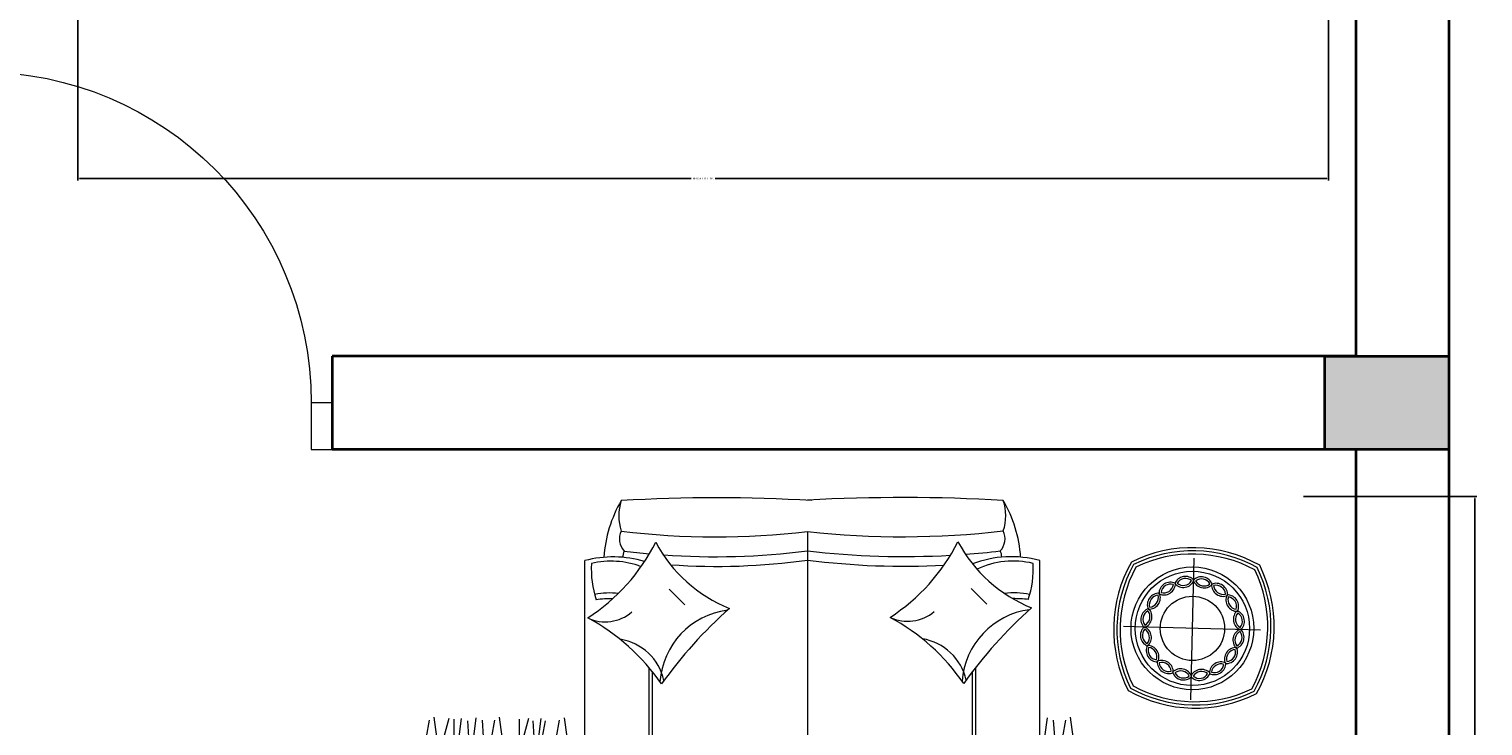
# Model space of a CAD drawing. Units: inches. Extents: x 1602 to 2642, y 1463 to 2270.
# Tile 3 of 5: x 1854 to 1995, y 1851 to 1919. Entities that reach past the tile are written whole.
import ezdxf

# ---------------------------------------------------------------- set-up
doc = ezdxf.new("R2010")
doc.units = ezdxf.units.IN
for name, color, linetype, lineweight in [('A-ANNO-DIMS', 2, 'Continuous', 18), ('A-COLS', 7, 'Continuous', 35), ('A-DOOR', 3, 'Continuous', 18), ('A-FURN', 8, 'Continuous', 13), ('A-WALL', 7, 'Continuous', 35)]:
    doc.layers.add(name, color=color, linetype=linetype, lineweight=lineweight)
doc.styles.get("Standard").update_dxf_attribs({"font": 'arial.ttf'})
doc.dimstyles.get("Standard").update_dxf_attribs({"dimtxt": 0.18, "dimasz": 0.18, "dimexe": 0.18, "dimexo": 0.0625, "dimgap": 0.09, "dimtad": 0, "dimtih": 1, "dimtoh": 1, "dimdec": 4, "dimzin": 0, "dimdsep": 46, "dimtxsty": 'Standard', "dimcen": 0.09, "dimadec": 0, "dimazin": 0, "dimtfac": 1, "dimtdec": 4, "dimtofl": 0, "dimtmove": 0, "dimatfit": 3, "dimfxl": 1, "dimtolj": 1, "dimtzin": 0, "dimarcsym": 0})

# ---------------------------------------------------------------- blocks, each defined once
blk = doc.blocks.new('A$C25EC1EFB')
for p, q in [((661.4278893405954, 627.3733247221026), (653.8786500493316, 683.1990086844235)), ((675.1174403770947, 635.1904524639612), (683.8521758037404, 683.1990086844235)), ((710.3189624152092, 635.1904524639612), (707.0057324760364, 683.1990086844235)), ((727.9198137478397, 629.3276369100713), (735.4071355219075, 683.1990086844235)), ((748.7809110632825, 692.29789009253), (748.7809110632752, 179.5278967396807)), ((932.0574757677549, 485.7876167851136), (932.0574757677622, 677.7735139828656)), ((941.2187188779444, 497.6639532491608), (941.2187188779517, 677.7735139828656)), ((1411.721483672338, 178.5414486224835), (1411.72148367236, 698.1899957858185)), ((1855.231064631016, 496.5022021999393), (1855.231064631016, 678.2458862606654)), ((1864.392307741191, 485.3713467841807), (1864.392307741191, 678.2458862606654)), ((2047.668872445676, 692.7702623703298), (2047.668872445669, 180.000269017466)), ((2106.284257832041, 629.3276369100713), (2098.999297799186, 683.1990086844235)), ((2120.382168021439, 635.1904524639612), (2129.116903448099, 683.1990086844235)), ((2160.816511778532, 637.1447646519445), (2169.195677255848, 683.1990086844235)), ((2172.776182239308, 631.2819490980546), (2179.991883601353, 683.1990086844235)), ((2196.018033816647, 637.1447646519445), (2192.839677453398, 683.1990086844235)), ((2207.977704277422, 631.2819490980546), (2222.476230384819, 683.1990086844235)), ((2235.131036778053, 633.2362612860233), (2235.131036778061, 683.1990086844235)), ((2291.844710444959, 627.3733247221026), (2284.295471153695, 683.1990086844235)), ((2305.534261481458, 635.1904524639612), (2314.268996908111, 683.1990086844235)), ((2340.735783519573, 635.1904524639612), (2337.422553580407, 683.1990086844235)), ((2358.336634852203, 629.3276369100713), (2365.823956626271, 683.1990086844235)), ((2382.548981739441, 637.1447646519445), (2379.370625376192, 683.1990086844235)), ((2400.149833072079, 631.2819490980546), (2407.365534434132, 683.1990086844235)), ((2421.66198470087, 633.2362612860233), (2421.66198470087, 683.1990086844235)), ((2435.351355110193, 631.2819490980546), (2449.849881217597, 683.1990086844235)), ((2478.375658367768, 627.3733247221026), (2470.826419076511, 683.1990086844235)), ((2492.065209404253, 635.1904524639612), (2500.799944830906, 683.1990086844235)), ((317.5955949916479, 577.5656340500936), (307.6667150012017, 173.5231372566268)), ((117.9581545735291, 378.2725583521751), (509.944476949613, 368.6399449918172)), ((944.1569903229192, 260.1207764131323), (899.4936078262272, 304.7423657605905)), ((1806.979157015697, 261.5530158658585), (1762.315774518969, 306.1746052133312)), ((1411.721483672338, 97.03052564927928), (1411.721483672338, 178.5414486224835))]:
    blk.add_line(p, q)
for radius in [175.3148329503734, 163.2405281737082, 91.75760778478207, 91.75760778478207]:
    blk.add_circle((312.7783746963924, 373.5789015934788), radius)
for centre, radius, start, end in [((304.5060052362623, 211.8475565177578), 389.4856216215981, 60.51981844412023, 116.664792315698), ((304.5060052362623, 211.8475565177578), 380.3212540540306, 60.94048126723747, 116.2441294929664), ((304.5060052362623, 211.8475565177578), 371.1568864864629, 61.3829579467198, 115.8016528138425), ((468.7739130891368, 368.2357101904127), 389.4856216216183, 150.5198184440689, 206.6647923151855), ((468.7739130891368, 368.2357101904127), 380.3212540540507, 150.940481267197, 206.2441294932469), ((468.7739130891368, 368.2357101904127), 371.1568864864831, 151.3829579460627, 205.8016528138911), ((148.1178515636002, 376.1154643706323), 380.3212540540452, 330.940481267197, 26.24412949324692), ((148.1178515636002, 376.1154643706323), 389.4856216216128, 330.519818444069, 26.66479231518558), ((249.9997773948071, 472.7989032444529), 32.81996572270785, 64.15706611601946, 180.4877419729194), ((231.4874083348714, 502.0572391685782), 32.81996572270785, 244.1570661160195, 0.4877419729194889), ((249.9997773948071, 472.7989032444529), 27.09223599297813, 72.03860713209241, 172.6062009563627), ((231.4874083348714, 502.0572391685782), 27.09223599297813, 252.0386071320924, 352.6062009563627), ((292.7483643607866, 489.2705594289509), 32.81996572270785, 41.65706611607041, 157.9877419721565), ((286.8418459047189, 523.3861140776643), 32.81996572270785, 221.6570661160704, 337.9877419721565), ((292.7483643607866, 489.2705594289509), 27.09223599297813, 49.53860713232503, 150.106200956097), ((286.8418459047189, 523.3861140776643), 27.09223599297813, 229.5386071323251, 330.106200956097), ((338.5463388277367, 488.1292094555174), 32.81996572270785, 19.15706611564963, 135.4877419728042), ((346.1448848678137, 521.9081988918551), 32.81996572270785, 199.1570661156496, 315.4877419728042), ((338.5463388277367, 488.1292094555174), 27.09223599297813, 27.03860713130998, 127.6062009564518), ((346.1448848678137, 521.9081988918551), 27.09223599297813, 207.03860713131, 307.6062009564517), ((400.3681751255808, 497.8484928007747), 32.81996572270785, 176.6570661157543, 292.9877419724641), ((380.4213743429809, 469.5486135112369), 32.81996572270785, 356.6570661157543, 112.9877419724641), ((148.1178515636002, 376.1154643706323), 371.1568864864776, 331.3829579460627, 25.80165281389105), ((-89.79630682914105, 1283.503210788018), 1296.354628148881, 311.6592367379425, 324.5116366281615), ((748.6744994247146, 540.2574918194805), 221.9945356540506, 277.5079417686749, 355.9655471801815), ((1107.71901087749, 554.2062067962761), 152.68412196255, 192.5229511730869, 261.0221639720215), ((1462.268417562738, 872.452021107798), 602.6484764389724, 214.5216399527675, 241.6492334140671), ((773.0258598636301, 1284.935450240729), 1296.354628148881, 311.6592367379425, 324.5116366281615), ((1611.496666117486, 541.6897312721921), 221.9945356540506, 277.5079417686749, 355.9655471801815), ((1970.541177570259, 555.6384462489732), 152.68412196255, 192.5229511730869, 261.0221639720215), ((2325.0905842555, 873.8842605605096), 602.6484764389724, 214.5216399527675, 241.6492334140671), ((216.8086627786706, 441.2219012401838), 32.81996572270785, 86.65706611574215, 202.9877419731067), ((188.5087834891474, 461.1687020227036), 32.81996572270785, 266.6570661157422, 22.98774197310666), ((216.8086627786706, 441.2219012401838), 27.09223599297813, 94.53860713211645, 195.1062009565991), ((188.5087834891474, 461.1687020227036), 27.09223599297813, 274.5386071321164, 15.1062009565991), ((380.4213743429809, 469.5486135112369), 27.09223599297813, 4.538607132124711, 105.1062009564984), ((400.3681751255808, 497.8484928007747), 27.09223599297813, 184.5386071321247, 285.1062009564985), ((441.2567122714627, 454.8698679549634), 32.81996572270785, 154.1570661158802, 270.4877419729204), ((411.99837634733, 436.357498895064), 32.81996572270785, 334.1570661158802, 90.48774197292038), ((441.2567122714627, 454.8698679549634), 27.09223599297813, 162.0386071315967, 262.6062009563761), ((411.99837634733, 436.357498895064), 27.09223599297813, 342.0386071315967, 82.60620095637618), ((198.228066834361, 399.3468657249396), 32.81996572270785, 109.1570661156154, 225.4877419725107), ((198.228066834361, 399.3468657249396), 27.09223599297813, 117.0386071317286, 217.6062009569093), ((164.4490773980596, 406.9454117649947), 32.81996572270785, 289.1570661156154, 45.4877419725107), ((164.4490773980596, 406.9454117649947), 27.09223599297813, 297.0386071317287, 37.60620095690924), ((462.5855871805706, 399.5154303851814), 32.81996572270785, 131.6570661153347, 247.9877419725821), ((462.5855871805706, 399.5154303851814), 27.09223599297813, 139.5386071315111, 240.1062009565103), ((428.4700325318499, 393.608911929121), 32.81996572270785, 311.6570661153347, 67.9877419725821), ((428.4700325318499, 393.608911929121), 27.09223599297813, 319.5386071315111, 60.10620095651037), ((197.0867168608983, 353.5488912579385), 32.81996572270785, 131.6570661153347, 247.9877419725821), ((162.9711622121776, 347.6423728018635), 32.81996572270785, 311.6570661153347, 67.9877419725821), ((197.0867168608983, 353.5488912579385), 27.09223599297813, 139.5386071315111, 240.1062009565103), ((162.9711622121776, 347.6423728018635), 27.09223599297813, 319.5386071315111, 60.10620095651037), ((461.1076719946304, 340.2123914221229), 32.81996572270785, 109.1570661156154, 225.4877419725107), ((461.1076719946304, 340.2123914221229), 27.09223599297813, 117.0386071317286, 217.6062009569093), ((427.3286825583218, 347.8109374621636), 32.81996572270785, 289.1570661156154, 45.4877419725107), ((427.3286825583218, 347.8109374621636), 27.09223599297813, 297.0386071317287, 37.60620095690924), ((1476.768636050912, -122.814034694944), 553.6612235346786, 122.8931183194097, 153.2777550472848), ((1126.024828213625, 236.6446309555395), 116.724496395002, 64.60120848363609, 130.5451974888048), ((2339.59080274366, -121.3817952422323), 553.6612235346786, 122.8931183194097, 153.2777550472848), ((1988.846994906402, 238.0768704082657), 116.724496395002, 64.60120848363609, 130.5451974888048), ((213.5583730454182, 310.8003042919372), 32.81996572270785, 154.1570661158802, 270.4877419729204), ((184.3000371212856, 292.2879352319942), 32.81996572270785, 334.1570661158802, 90.48774197292038), ((213.5583730454182, 310.8003042919372), 27.09223599297813, 162.0386071315967, 262.6062009563761), ((184.3000371212856, 292.2879352319942), 27.09223599297813, 342.0386071315967, 82.60620095637618), ((437.0479659035136, 285.9891011644868), 32.81996572270785, 86.65706611574215, 202.9877419731067), ((408.7480866139831, 305.9359019470648), 32.81996572270785, 266.6570661157422, 22.98774197310666), ((437.0479659035136, 285.9891011644868), 27.09223599297813, 94.53860713211645, 195.1062009565991), ((408.7480866139831, 305.9359019470648), 27.09223599297813, 274.5386071321164, 15.1062009565991), ((1041.47230199355, 204.3337353688039), 274.1566884687789, 161.5150475002156, 183.3971191000656), ((618.930007287834, -66.98351007430028), 411.4538102731095, 27.99465948751157, 68.17621387936651), ((821.4386098706109, 598.0218173387474), 309.3592482736565, 262.5749152314042, 270.8047485918586), ((1481.752173980598, -65.55127062158863), 411.4538102731095, 27.99465948751157, 68.17621387936651), ((1975.011173638355, 598.4941896165473), 309.3592482736565, 268.7325582962257, 277.4250847685958), ((1754.97748151541, 204.8061076465892), 274.1566884687789, 356.6028808999344, 18.48495249978436), ((245.1353750497019, 277.6091896758808), 32.81996572270785, 176.6570661157543, 292.9877419724641), ((225.1885742671675, 249.309310386343), 32.81996572270785, 356.6570661157543, 112.9877419724641), ((225.1885742671675, 249.309310386343), 27.09223599297813, 4.538607132124711, 105.1062009564984), ((245.1353750497019, 277.6091896758808), 27.09223599297813, 184.5386071321247, 285.1062009564985), ((279.4118645249128, 225.2496042952771), 32.81996572270785, 19.15706611564963, 135.4877419728042), ((279.4118645249128, 225.2496042952771), 27.09223599297813, 27.03860713130998, 127.6062009564518), ((338.7149034880658, 223.7716891095115), 32.81996572270785, 41.65706611607041, 157.9877419721565), ((338.7149034880658, 223.7716891095115), 27.09223599297813, 49.53860713232503, 150.106200956097), ((394.0693410578406, 245.1005640184521), 32.81996572270785, 64.15706611601946, 180.4877419729194), ((375.5569719979121, 274.358899942592), 32.81996572270785, 244.1570661160195, 0.4877419729194889), ((394.0693410578406, 245.1005640184521), 27.09223599297813, 72.03860713209241, 172.6062009563627), ((375.5569719979121, 274.358899942592), 27.09223599297813, 252.0386071320924, 352.6062009563627), ((821.9997660819736, 497.8256545033873), 225.8008880027097, 258.6738781626161, 277.0247756611929), ((1974.450017426992, 498.2980267811872), 225.8008880027097, 264.2072358022266, 281.3261218373839), ((287.0104105649825, 259.0285937316148), 32.81996572270785, 199.1570661156496, 315.4877419728042), ((287.0104105649825, 259.0285937316148), 27.09223599297813, 207.03860713131, 307.6062009564517), ((332.8083850320272, 257.8872437582395), 32.81996572270785, 221.6570661160704, 337.9877419721565), ((332.8083850320272, 257.8872437582395), 27.09223599297813, 229.5386071323251, 330.106200956097), ((312.3857594164747, 532.5036180433016), 389.4856216216215, 240.5198184441202, 296.664792315698), ((312.3857594164747, 532.5036180433016), 380.321254054054, 240.9404812672375, 296.2441294929665), ((312.3857594164747, 532.5036180433016), 371.1568864864865, 241.3829579467198, 295.8016528138426), ((829.5512177542569, 485.6793434299543), 316.6268320175827, 255.2207135339614, 290.5803261072686), ((824.5552444838121, 418.6445313216027), 237.4397884308417, 256.1700435482352, 295.7780897744407), ((1175.131801040306, 195.6787475668607), 372.842184662441, 183.9255453890698, 210.1803651628055), ((896.7352778358709, 170.0316774215971), 39.55947945866067, 179.6693879436746, 206.2356847376864), ((1134.712812991691, -2188.905712423344), 2357.364478536592, 83.25170869535147, 93.18633975577367), ((1138.003293432486, -1934.098548346105), 2130.205316173485, 82.61743616467076, 93.12234043389631), ((1671.190347158454, -1678.660801258542), 1875.239794821453, 85.97990558961646, 97.95328726902667), ((1676.501174276864, -1941.592820043814), 2110.523956920629, 86.01035178291525, 97.20713913467989), ((1966.898565754723, 486.1517157077396), 316.6268320175827, 253.4758498435309, 284.7792864660386), ((1971.894539025154, 419.1169035994025), 237.4397884308417, 249.0286919001191, 283.8299564517648), ((1899.714505673104, 170.504049699397), 39.55947945866067, 333.7643152623136, 0.3306120563253654), ((1621.317982468661, 196.151119844646), 372.842184662441, 329.8196348371945, 356.0744546109302), ((899.5691667209556, 117.6234067020195), 51.84314058293741, 137.6561394551597, 205.6360597976045), ((1134.712812991691, -2188.905712423344), 2357.364478536592, 94.23182541585733, 96.66148904496858), ((1676.501174276864, -1941.592820043814), 2110.523956920629, 82.95926216841848, 84.92619671585597), ((1896.880616788012, 118.0957789798049), 51.84314058293741, 334.3639402023955, 42.3438605448403), ((980.6545422172584, 51.71771758796968), 135.0162301971975, 161.2159189721368, 198.7840810278632), ((1139.803975331213, -2360.101508648899), 2472.008696990425, 83.684764843546, 96.6664762080601), ((1672.028446620878, -2102.590796459226), 2214.970355475213, 82.95686810056368, 96.74909123360197), ((1815.795241291709, 52.19008986576955), 135.0162301971975, 341.2159189721368, 18.78408102786323), ((1139.805526238788, 4996.653274943332), 4996.658984712837, 266.7074856531846, 273.1195518594664), ((1671.435778389403, 4495.731419435651), 4495.264757303411, 266.5286646494081, 273.4713353505918)]:
    blk.add_arc(centre, radius, start, end)
blk = doc.blocks.new('DOOR-SWING-32IN')
for p, q in [((32.5, 4.500000000000227), (32.5, 36.46482441684952)), ((34, 4.500000000000227), (34, 36.50000000000023)), ((0, 4.500000000000454), (2, 4.500000000000454)), ((2, 4.500000000000454), (2, 4.547e-13)), ((34, 4.500000000000227), (32.5, 4.500000000000227)), ((36, 4.500000000000454), (34, 4.500000000000454)), ((34, 4.500000000000454), (34, 4.547e-13)), ((2, 4.547e-13), (0, 6.821e-13)), ((34, 4.547e-13), (36, 6.821e-13))]:
    blk.add_line(p, q)
blk.add_arc((34, 4.500000000000454), 31.99999999999977, 90, 180)
blk = doc.blocks.new('COL-12X9')
h = blk.add_hatch(color=256)
h.dxf.hatch_style = 1
h.paths.add_polyline_path([(11.99999999999977, 4.547e-13), (11.99999999999977, 9.000000000000455), (-2.274e-13, 9.000000000000455), (-2.274e-13, 4.547e-13)])
blk.add_lwpolyline([(11.99999999999977, 9.000000000000455), (11.99999999999977, 4.547e-13), (-2.274e-13, 4.547e-13), (-2.274e-13, 9.000000000000455)], close=True)
blk = doc.blocks.new('*D15')
at = {"layer": 'A-ANNO-DIMS', "color": 0, "lineweight": -2, "transparency": 16777216}
for p, q in [((1859.139100534901, 1922.525713110817), (1859.139100534901, 1904.263418151082)), ((1980.104400266467, 1922.525713110817), (1980.104400266467, 1904.263418151082)), ((1859.319100534901, 1904.443418151082), (1918.454819977765, 1904.443418151082)), ((1979.924400266467, 1904.443418151082), (1920.788680823603, 1904.443418151082))]:
    blk.add_line(p, q, dxfattribs=at)
at = {"layer": 'A-ANNO-DIMS', "color": 0, "transparency": 16777216}
for points in [[(1859.319100534901, 1904.473418151082), (1859.319100534901, 1904.413418151082), (1859.139100534901, 1904.443418151082)], [(1979.924400266467, 1904.473418151082), (1979.924400266467, 1904.413418151082), (1980.104400266467, 1904.443418151082)]]:
    blk.add_solid(points, dxfattribs=at)
at = {"layer": 'Defpoints', "color": 0, "transparency": 16777216}
for p in [(1859.139100534901, 1922.588213110817), (1980.104400266467, 1922.588213110817), (1980.104400266467, 1904.443418151082)]:
    blk.add_point(p, dxfattribs=at)
at = {"layer": 'A-ANNO-DIMS', "color": 0, "transparency": 16777216, "insert": (1919.621750400684, 1904.443418151082), "char_height": 0.18, "attachment_point": 5}
blk.add_mtext('\\A1;BED SET 121 TYP.', dxfattribs=at)
blk = doc.blocks.new('*D19')
at = {"layer": 'A-ANNO-DIMS', "color": 0, "lineweight": -2, "transparency": 16777216}
for p, q in [((1977.681887442998, 1873.678767726278), (1994.435915796376, 1873.678767726278)), ((1994.255915796377, 1873.498767726278), (1994.255915796377, 1818.406804183643)), ((1994.255915796377, 1762.948578703764), (1994.255915796377, 1818.040542246398)), ((1977.681887442998, 1762.768578703764), (1994.435915796376, 1762.768578703764))]:
    blk.add_line(p, q, dxfattribs=at)
at = {"layer": 'A-ANNO-DIMS', "color": 0, "transparency": 16777216}
for points in [[(1994.225915796377, 1873.498767726278), (1994.285915796377, 1873.498767726278), (1994.255915796377, 1873.678767726278)], [(1994.225915796377, 1762.948578703764), (1994.285915796377, 1762.948578703764), (1994.255915796377, 1762.768578703764)]]:
    blk.add_solid(points, dxfattribs=at)
at = {"layer": 'Defpoints', "color": 0, "transparency": 16777216}
for p in [(1977.619387442998, 1873.678767726278), (1977.619387442998, 1762.768578703764), (1994.255915796377, 1762.768578703764)]:
    blk.add_point(p, dxfattribs=at)
at = {"layer": 'A-ANNO-DIMS', "color": 0, "transparency": 16777216, "insert": (1994.255915796377, 1818.22367321502), "char_height": 0.18, "attachment_point": 5}
blk.add_mtext('\\A1;SOFA SET 111', dxfattribs=at)

msp = doc.modelspace()

# ---------------------------------------------------------------- linework, layer by layer
at = {"layer": 'A-WALL'}
for p, q in [((1991.726933683589, 2040.248102623293), (1991.726933683589, 1725.248102623292)), ((1982.726933683589, 2031.248102623293), (1982.726933683589, 1887.248102623292)), ((1982.72693368359, 1887.248102623292), (1883.726933683589, 1887.248102623292)), ((1883.726933683589, 1887.248102623292), (1883.726933683589, 1878.248102623292)), ((1982.72693368359, 1878.248102623292), (1883.726933683589, 1878.248102623292)), ((1982.726933683589, 1878.248102623292), (1982.726933683589, 1725.248102623293))]:
    msp.add_line(p, q, dxfattribs=at)

# ---------------------------------------------------------------- block references
at = {"layer": 'A-COLS'}
msp.add_blockref('COL-12X9', (1979.726933683589, 1878.248102623292), dxfattribs=at)
at = {"layer": 'A-DOOR', "extrusion": (0, 0, -1), "zscale": -1}
msp.add_blockref('DOOR-SWING-32IN', (-1883.726933683589, 1878.248102623292), dxfattribs=at)
at = {"layer": 'A-FURN', "xscale": 0.0338700972235775, "yscale": 0.0338700972235775, "zscale": 0.0338700972235775, "rotation": 180}
msp.add_blockref('A$C25EC1EFB', (1977.526265282426, 1873.585705524922), dxfattribs=at)

# ---------------------------------------------------------------- dimensions: what is measured, and where the dimension line sits
at = {"layer": 'A-ANNO-DIMS'}
dim = msp.add_linear_dim(base=(1980.104400266467, 1904.443418151082), p1=(1859.139100534901, 1922.588213110817), p2=(1980.104400266467, 1922.588213110817), text='BED SET <> TYP.', dimstyle='Standard', override={"dimdec": 0, "dimlfac": 1, "dimrnd": 0, "dimzin": 0, "dimdsep": 46, "dimlunit": 2}, dxfattribs=at)
dim.commit()
dim.dimension.update_dxf_attribs({"geometry": '*D15', "text_midpoint": (1919.621750400684, 1904.443418151082)})
dim = msp.add_linear_dim(base=(1994.255915796377, 1762.768578703764), p1=(1977.619387442997, 1873.678767726277), p2=(1977.619387442997, 1762.768578703763), angle=270, text='SOFA SET <>', dimstyle='Standard', override={"dimdec": 0, "dimlfac": 1, "dimrnd": 0, "dimzin": 0, "dimdsep": 46, "dimlunit": 2}, dxfattribs=at)
dim.commit()
dim.dimension.update_dxf_attribs({"geometry": '*D19', "text_midpoint": (1994.255915796377, 1818.22367321502)})

doc.saveas('drawing.dxf')
